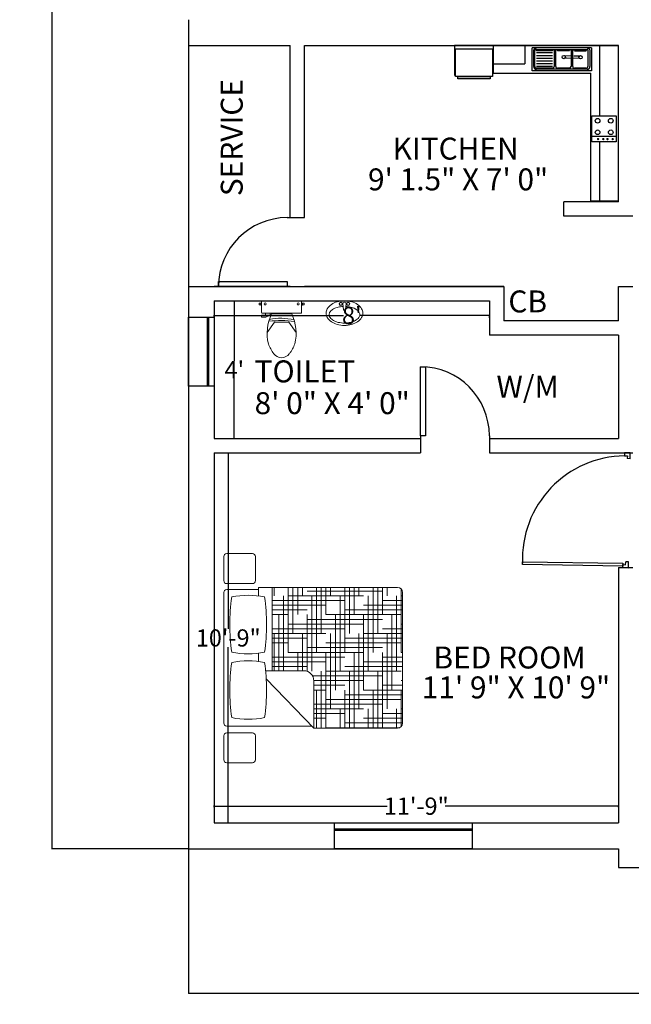
# Model space of a CAD drawing. Units: inches. Extents: x -113 to 5399, y -1393 to 3302.
# Tile 23 of 40: x 3631 to 3844, y -154 to 189. Entities that reach past the tile are written whole.
import ezdxf

# ---------------------------------------------------------------- set-up
doc = ezdxf.new("R2010")
doc.units = ezdxf.units.IN
doc.header["$MEASUREMENT"] = 0
for name, color, linetype, lineweight in [('A-ANNO-DIMS', 254, 'Continuous', 18), ('A-AREA-IDEN', 4, 'Continuous', 18), ('A-FLOR-CASE', 8, 'Continuous', 18), ('A-FLOR-FIXT', 8, 'Continuous', 18), ('doors', 2, 'Continuous', 25), ('DT TEXT', 4, 'Continuous', 18), ('furniture', 131, 'Continuous', 18), ('walls', 1, 'Continuous', 25), ('windows', 3, 'Continuous', 25)]:
    doc.layers.add(name, color=color, linetype=linetype, lineweight=lineweight)
doc.layers.add('A-GLAZ-PATT', color=85, linetype='Continuous', lineweight=13, true_color=0x58ba48)
doc.layers.add('TEFRIŞ', color=11, linetype='Continuous')
doc.styles.get("Standard").update_dxf_attribs({"font": 'arial.ttf'})
doc.dimstyles.get("Standard").update_dxf_attribs({"dimtxt": 6, "dimasz": 0.18, "dimexe": 0.18, "dimexo": 0.0625, "dimgap": 0.09, "dimtad": 0, "dimtih": 1, "dimtoh": 1, "dimdec": 1, "dimzin": 0, "dimdsep": 46, "dimlunit": 4, "dimtxsty": 'Standard', "dimblk": 'ARCHTICK', "dimcen": 0.09, "dimadec": 0, "dimazin": 0, "dimtfac": 1, "dimtdec": 1, "dimtofl": 0, "dimtmove": 0, "dimatfit": 3, "dimfxl": 1, "dimtolj": 1, "dimtzin": 0, "dimarcsym": 0})

# ---------------------------------------------------------------- blocks, each defined once
blk = doc.blocks.new('*U2')
for p, q in [((0, 0), (0, -6)), ((24, 0), (24, -6))]:
    blk.add_line(p, q)
blk.add_lwpolyline([(0, 0), (0, 24), (1.75, 24), (1.75, 0)], close=True)
blk.add_arc((0, 0), 24, 0, 90)
blk = doc.blocks.new('*X4')
at = {"color": 0}
for p, q in [((4.3594, 18.5625), (4.3594, 18.6457)), ((4.5, 18), (4.5, 18.6457)), ((4.5469, 18.1875), (4.5469, 18.6457)), ((4.5938, 18.375), (4.5938, 18.6457)), ((4.6406, 18.5625), (4.6406, 18.6457)), ((4.7812, 18), (4.7812, 18.6457)), ((4.8281, 18.1875), (4.8281, 18.6457)), ((4.875, 18.375), (4.875, 18.6457)), ((4.9219, 18.5625), (4.9219, 18.6457)), ((5.0625, 18), (5.0625, 18.6457)), ((5.1094, 18.1875), (5.1094, 18.6457)), ((5.1562, 18.375), (5.1562, 18.6457)), ((5.2031, 18.5625), (5.2031, 18.6457)), ((5.3438, 18), (5.3438, 18.6457)), ((5.3906, 18.1875), (5.3906, 18.6457)), ((5.4375, 18.375), (5.4375, 18.6457)), ((5.4844, 18.5625), (5.4844, 18.6457)), ((5.625, 18), (5.625, 18.6287)), ((4.4531, 17.8169), (4.4531, 18.5625)), ((4.5, 18.5625), (5.25, 18.5625)), ((4.6875, 18.6094), (5.4375, 18.6094)), ((4.7344, 17.8125), (4.7344, 18.5625)), ((5.0156, 17.8125), (5.0156, 18.5625)), ((5.2969, 17.8125), (5.2969, 18.5625)), ((5.5781, 17.8125), (5.5781, 18.5625)), ((5.625, 18.5625), (5.6375, 18.5625)), ((4.3395, 18.5156), (5.0625, 18.5156)), ((4.3395, 18.4688), (4.875, 18.4688)), ((5.25, 18.4688), (5.6375, 18.4688)), ((5.4375, 18.5156), (5.6375, 18.5156)), ((4.3395, 18.4219), (4.6875, 18.4219)), ((4.3395, 18.375), (4.5, 18.375)), ((4.4062, 17.8169), (4.4062, 18.375)), ((4.6875, 17.8114), (4.6875, 18.375)), ((4.6875, 18.3281), (5.4375, 18.3281)), ((4.875, 18.375), (5.625, 18.375)), ((4.9688, 17.625), (4.9688, 18.375)), ((5.0625, 18.4219), (5.6375, 18.4219)), ((5.25, 17.625), (5.25, 18.375)), ((5.5312, 17.625), (5.5312, 18.375)), ((4.3395, 18.2344), (5.0625, 18.2344)), ((4.5, 18.2812), (5.25, 18.2812)), ((5.4375, 18.2344), (5.6375, 18.2344)), ((5.625, 18.2812), (5.6375, 18.2812)), ((4.3395, 18.1875), (4.875, 18.1875)), ((4.3395, 18.1406), (4.6875, 18.1406)), ((4.3594, 17.8169), (4.3594, 18.1875)), ((4.6406, 17.8169), (4.6406, 18.1875)), ((4.9219, 17.4375), (4.9219, 18.1875)), ((5.0625, 18.1406), (5.6375, 18.1406)), ((5.2031, 17.4375), (5.2031, 18.1875)), ((5.25, 18.1875), (5.6375, 18.1875)), ((5.4844, 17.4375), (5.4844, 18.1875)), ((4.3395, 18.0938), (4.5, 18.0938)), ((4.6875, 18.0469), (5.4375, 18.0469)), ((4.875, 18.0938), (5.625, 18.0938)), ((4.3395, 17.9531), (5.0625, 17.9531)), ((4.5, 18), (5.25, 18)), ((4.5938, 17.8169), (4.5938, 18)), ((4.875, 17.25), (4.875, 18)), ((5.1562, 17.25), (5.1562, 18)), ((5.4375, 17.25), (5.4375, 18)), ((5.4375, 17.9531), (5.6375, 17.9531)), ((5.625, 18), (5.6375, 18)), ((4.3395, 17.9062), (4.875, 17.9062)), ((4.3395, 17.8594), (4.6875, 17.8594)), ((5.0625, 17.8594), (5.6375, 17.8594)), ((5.25, 17.9062), (5.6375, 17.9062)), ((4.7421, 17.7656), (5.4375, 17.7656)), ((4.8281, 17.2457), (4.8281, 17.8125)), ((4.875, 17.8125), (5.625, 17.8125)), ((5.1094, 17.2457), (5.1094, 17.8125)), ((5.3906, 17.2457), (5.3906, 17.8125)), ((4.7548, 17.7188), (5.25, 17.7188)), ((4.7548, 17.6719), (5.0625, 17.6719)), ((5.4375, 17.6719), (5.6375, 17.6719)), ((5.625, 17.7188), (5.6375, 17.7188)), ((4.7548, 17.625), (4.875, 17.625)), ((4.7812, 17.2457), (4.7812, 17.625)), ((5.0625, 17.2457), (5.0625, 17.625)), ((5.0625, 17.5781), (5.6375, 17.5781)), ((5.25, 17.625), (5.6375, 17.625)), ((5.3438, 17.2457), (5.3438, 17.625)), ((5.625, 17.2627), (5.625, 17.625)), ((4.7548, 17.4844), (5.4375, 17.4844)), ((4.875, 17.5312), (5.625, 17.5312)), ((4.7548, 17.4375), (5.25, 17.4375)), ((4.7548, 17.3906), (5.0625, 17.3906)), ((5.0156, 17.2457), (5.0156, 17.4375)), ((5.2969, 17.2457), (5.2969, 17.4375)), ((5.4375, 17.3906), (5.6375, 17.3906)), ((5.5781, 17.2457), (5.5781, 17.4375)), ((5.625, 17.4375), (5.6375, 17.4375)), ((4.7548, 17.3438), (4.875, 17.3438)), ((4.875, 17.25), (5.6077, 17.25)), ((4.9688, 17.2457), (4.9688, 17.25)), ((5.0625, 17.2969), (5.6375, 17.2969)), ((5.25, 17.3438), (5.6375, 17.3438)), ((5.25, 17.2457), (5.25, 17.25)), ((5.5312, 17.2457), (5.5312, 17.25))]:
    blk.add_line(p, q, dxfattribs=at)
blk = doc.blocks.new('MAT-P01')
for p, q in [((-0.0213, 0.8164), (-0.0213, 0.5605)), ((0.0087, 0.8464), (0.2471, 0.8464)), ((0.2771, 0.8164), (0.2771, 0.5605)), ((0.3437, 0.8164), (0.3437, -0.0316)), ((0.3737, 0.8464), (1.6737, 0.8464)), ((1.7037, 0.8164), (1.7037, 0.5005)), ((1.7622, 0.8164), (1.7622, 0.5605)), ((1.7922, 0.8464), (2.0306, 0.8464)), ((2.0606, 0.8164), (2.0606, 0.5605)), ((0.0087, 0.5305), (0.2471, 0.5305)), ((0.9879, 0.5005), (1.0693, 0.5005)), ((1.6393, 0.5005), (1.7237, 0.5005)), ((1.7237, 0.5005), (1.7237, -0.8836)), ((1.7922, 0.5305), (2.0306, 0.5305)), ((0.8146, 0.423), (0.3237, -0.0509)), ((0.8949, 0.4293), (0.8949, 0.0491)), ((0.8949, 0.3643), (1.7237, 0.3643)), ((0.8949, 0.3643), (0.8949, 0.0491)), ((0.8949, 0.3643), (1.7237, 0.3643)), ((1.7237, 0.3643), (1.7237, -0.8836)), ((0.3237, -0.0509), (0.7949, -0.0509)), ((0.3237, -0.0509), (0.3237, -0.8836)), ((0.3737, -0.9336), (1.6737, -0.9336))]:
    blk.add_line(p, q)
for centre, radius, start, end in [((0.0087, 0.8164), 0.03, 90, 180), ((0.2471, 0.8164), 0.03, 0, 90), ((0.3737, 0.8164), 0.03, 90, 180), ((0.7029, -1.1436), 1.9306, 81.81622, 98.18378), ((1.3543, -1.1436), 1.9306, 81.81622, 98.18378), ((1.6737, 0.8164), 0.03, 0, 90), ((1.7922, 0.8164), 0.03, 90, 180), ((2.0306, 0.8164), 0.03, 0, 90), ((1.2251, 0.6034), 0.8138, 168.37298, 191.62702), ((0.1806, 0.6034), 0.8138, 348.37298, 11.62702), ((1.8766, 0.6034), 0.8138, 168.37298, 191.62702), ((0.8321, 0.6034), 0.8138, 348.37298, 11.62702), ((0.0087, 0.5605), 0.03, 180, 270), ((0.2471, 0.5605), 0.03, 270, 0), ((1.7922, 0.5605), 0.03, 180, 270), ((2.0306, 0.5605), 0.03, 270, 0), ((0.7029, 2.3504), 1.9306, 261.81622, 278.18378), ((1.3543, 2.3504), 1.9306, 261.81622, 278.18378), ((0.7949, 0.0491), 0.1, 270, 0), ((0.3737, -0.8836), 0.05, 180, 270), ((1.6737, -0.8836), 0.05, 270, 0)]:
    blk.add_arc(centre, radius, start, end)
at = {"rotation": 270}
blk.add_blockref('*X4', (-16.9221, 4.7038), dxfattribs=at)
blk = doc.blocks.new('A$C008029BD')
at = {"layer": 'TEFRIŞ', "ltscale": 0.05}
for p, q in [((0, 0), (0, -3.55)), ((3.37, 0), (0, 0)), ((3.37, 0), (3.37, -0.6)), ((1.522, -0.4), (0, -0.4)), ((3.37, -0.4), (2.083, -0.4)), ((0.05, -0.581), (0.05, -1.869)), ((0.05, -0.581), (0.55, -0.581)), ((0.096, -0.617), (0.454, -0.617)), ((0.55, -0.581), (0.55, -1.869)), ((0.6, -2.71), (0.6, -0.6)), ((3.37, -0.6), (0.6, -0.6)), ((0.086, -1.773), (0.086, -0.677)), ((0.099, -0.659), (0.457, -0.659)), ((0.113, -0.954), (0.113, -0.695)), ((0.23, -0.846), (0.229, -0.967)), ((0.28, -0.846), (0.277, -1.158)), ((0.493, -0.695), (0.493, -0.954)), ((0.514, -0.677), (0.514, -1.773)), ((0.096, -1.024), (0.454, -1.024)), ((0.457, -0.99), (0.099, -0.99)), ((0.11, -1.319), (0.11, -1.06)), ((0.228, -1.02), (0.227, -1.159)), ((0.49, -1.06), (0.49, -1.319)), ((0.454, -1.355), (0.096, -1.355)), ((0.096, -1.391), (0.454, -1.391)), ((0.11, -1.773), (0.11, -1.427)), ((0.154, -1.773), (0.154, -1.427)), ((0.214, -1.773), (0.214, -1.427)), ((0.274, -1.773), (0.274, -1.427)), ((0.334, -1.773), (0.334, -1.427)), ((0.39, -1.773), (0.39, -1.427)), ((0.444, -1.773), (0.444, -1.427)), ((0.49, -1.427), (0.49, -1.773)), ((0.55, -1.869), (0.05, -1.869)), ((0.454, -1.809), (0.096, -1.809)), ((0.454, -1.833), (0.096, -1.833)), ((0, -2.025), (0.4, -2.025)), ((0.4, -2.71), (0.4, -2.025)), ((0, -2.71), (0.6, -2.71)), ((0, -3.55), (0.65, -3.55))]:
    blk.add_line(p, q, dxfattribs=at)
at = {"layer": 'TEFRIŞ'}
blk.add_line((1.969, -0.05), (1.969, -0.572), dxfattribs=at)
at = {"layer": 'TEFRIŞ', "ltscale": 0.05}
for points in [[(1.522, -0.05), (2.083, -0.05), (2.083, -0.572), (1.522, -0.572)], [(0.67, -2.73), (0.67, -3.53), (0.07, -3.53), (0.07, -2.73)], [(0.72, -2.78), (0.72, -3.48), (0.67, -3.48), (0.67, -2.78)]]:
    blk.add_lwpolyline(points, close=True, dxfattribs=at)
at = {"layer": 'TEFRIŞ', "const_width": 0.025}
for points in [[(2.014, -0.123, 1), (2.039, -0.123, 1)], [(2.014, -0.236, 1), (2.039, -0.236, 1)], [(2.014, -0.327, 1), (2.039, -0.327, 1)], [(2.014, -0.44, 1), (2.039, -0.44, 1)]]:
    blk.add_lwpolyline(points, format="xyb", close=True, dxfattribs=at)
at = {"layer": 'TEFRIŞ', "ltscale": 0.05}
for centre, radius in [((1.628, -0.164), 0.0505), ((1.628, -0.45), 0.0505), ((0.255, -0.82), 0.036), ((0.252, -1.184), 0.036)]:
    blk.add_circle(centre, radius, dxfattribs=at)
at = {"layer": 'TEFRIŞ'}
for centre in [(1.88, -0.164), (1.88, -0.45)]:
    blk.add_circle(centre, 0.0505, dxfattribs=at)
at = {"layer": 'TEFRIŞ', "ltscale": 0.05}
for centre, radius, start, end in [((0.108, -0.649), 0.0351, 110.4976, 230.5777), ((0.454, -0.677), 0.06, 0, 90), ((0.118, -0.673), 0.023, 143.9853, 258.5157), ((0.457, -0.695), 0.036, 0, 90), ((0.115, -1.038), 0.023, 143.9853, 258.5157), ((0.118, -0.976), 0.023, 101.4843, 216.0147), ((0.454, -1.06), 0.036, 0, 90), ((0.457, -0.954), 0.036, 270, 0), ((0.115, -1.341), 0.023, 101.4843, 216.0147), ((0.115, -1.405), 0.023, 143.9853, 258.5157), ((0.454, -1.319), 0.036, 270, 0), ((0.454, -1.427), 0.036, 0, 90), ((0.108, -1.801), 0.0351, 129.4223, 249.5024), ((0.115, -1.796), 0.023, 101.4843, 216.0147), ((0.454, -1.773), 0.06, 270, 0), ((0.454, -1.773), 0.036, 270, 0)]:
    blk.add_arc(centre, radius, start, end, dxfattribs=at)
blk = doc.blocks.new('toilet-3')
at = {"color": 0, "linetype": 'ByBlock'}
for p, q in [((-0.281, -0.05), (-0.281, -0.069)), ((-0.281, -0.05), (-0.261, -0.05)), ((-0.281, -0.069), (-0.261, -0.069)), ((-0.261, -0.047), (-0.261, -0.072)), ((-0.261, -0.047), (-0.251, -0.047)), ((-0.261, -0.072), (-0.251, -0.072)), ((-0.251, -0.047), (-0.251, -0.072)), ((-0.25, -0.03), (-0.25, -0.165)), ((0.24, -0.02), (-0.24, -0.02)), ((0.25, -0.03), (0.25, -0.165)), ((0.261, -0.047), (0.251, -0.047)), ((0.251, -0.047), (0.251, -0.072)), ((0.261, -0.072), (0.251, -0.072)), ((0.261, -0.047), (0.261, -0.072)), ((0.281, -0.05), (0.261, -0.05)), ((0.281, -0.069), (0.261, -0.069)), ((0.281, -0.05), (0.281, -0.069)), ((-0.144, -0.2), (-0.25, -0.2)), ((-0.25, -0.2), (-0.25, -0.222)), ((-0.198, -0.222), (-0.25, -0.222)), ((0.24, -0.175), (-0.24, -0.175)), ((-0.202, -0.2), (-0.202, -0.175)), ((-0.198, -0.222), (-0.16, -0.207)), ((-0.16, -0.207), (-0.16, -0.2)), ((-0.144, -0.2), (-0.144, -0.175)), ((0.125, -0.182), (-0.125, -0.182)), ((-0.089, -0.287), (-0.18, -0.415)), ((0.089, -0.287), (-0.089, -0.287)), ((0.089, -0.287), (0.18, -0.415))]:
    blk.add_line(p, q, dxfattribs=at)
for centre in [(-0.205, -0.059), (0.205, -0.059)]:
    blk.add_circle(centre, 0.0125, dxfattribs=at)
for centre, radius, start, end in [((-0.24, -0.03), 0.01, 90, 180), ((0.24, -0.03), 0.01, 0, 90), ((-0.24, -0.165), 0.01, 180, 270), ((0.376, -0.424), 0.557, 154.2321, 193.6755), ((-0.005, -0.896), 0.659, 75.9276, 103.0204), ((-0.376, -0.424), 0.557, 346.3245, 25.7679), ((0.24, -0.165), 0.01, 270, 0), ((-0.013, -1.787), 1.521, 83.4552, 95.5271), ((0.262, -0.406), 0.452, 199.2942, 217.2549), ((-0.265, -0.4), 0.457, 322.2382, 340.1051), ((-0.001, -0.609), 0.12, 216.3794, 323.6206)]:
    blk.add_arc(centre, radius, start, end, dxfattribs=at)
blk = doc.blocks.new('wash-6')
at = {"color": 0, "linetype": 'ByBlock'}
for p, q in [((-0.036, -0.063), (-0.021, -0.18)), ((0.036, -0.063), (0.021, -0.18))]:
    blk.add_line(p, q, dxfattribs=at)
for centre, radius in [((-0.075, -0.062), 0.0325), ((-0.075, -0.062), 0.0263), ((0.075, -0.062), 0.0325), ((0.075, -0.062), 0.0263)]:
    blk.add_circle(centre, radius, dxfattribs=at)
for centre, radius, start, end in [((0, -0.56), 0.56, 90, 105.4371), ((-0.204, -0.25), 0.17, 148.1465, 180), ((-0.107, -0.311), 0.285, 123.6901, 148.1465), ((-0.114, -0.361), 0.225, 118.369, 142.5096), ((-0.042, -0.407), 0.401, 105.4371, 123.6901), ((-0.045, -0.488), 0.37, 102.6081, 118.369), ((0, -0.69), 0.576, 92.9466, 102.6081), ((0, -0.063), 0.0361, 0, 180), ((0, -0.18), 0.0215, 180, 0), ((0, -0.56), 0.56, 74.5629, 90), ((0, -0.69), 0.576, 77.3919, 87.0534), ((0.045, -0.488), 0.37, 61.631, 77.3919), ((0.042, -0.407), 0.401, 56.3099, 74.5629), ((0.114, -0.361), 0.225, 37.4904, 61.631), ((0.107, -0.311), 0.285, 31.8535, 56.3099), ((0.204, -0.25), 0.17, 0, 31.8535), ((-0.204, -0.25), 0.17, 180, 211.8535), ((-0.107, -0.189), 0.285, 211.8535, 236.3099), ((-0.217, -0.282), 0.0954, 142.5096, 180), ((-0.217, -0.282), 0.0954, 180, 217.4904), ((-0.114, -0.203), 0.225, 217.4904, 241.631), ((0.114, -0.203), 0.225, 298.369, 322.5096), ((0.107, -0.189), 0.285, 303.6901, 328.1465), ((0.217, -0.282), 0.0954, 0, 37.4904), ((0.217, -0.282), 0.0954, 322.5096, 0), ((0.204, -0.25), 0.17, 328.1465, 0), ((-0.042, -0.092), 0.401, 236.3099, 254.5629), ((-0.045, -0.076), 0.37, 241.631, 257.3919), ((0, 0.06), 0.56, 254.5629, 270), ((0, 0.125), 0.576, 257.3919, 270), ((0, 0.125), 0.576, 270, 282.6081), ((0, 0.06), 0.56, 270, 285.4371), ((0.045, -0.076), 0.37, 282.6081, 298.369), ((0.042, -0.092), 0.401, 285.4371, 303.6901)]:
    blk.add_arc(centre, radius, start, end, dxfattribs=at)
blk = doc.blocks.new('_ArchTick')
at = {"color": 0, "linetype": 'ByBlock', "const_width": 0.15}
blk.add_lwpolyline([(-0.5, -0.5), (0.5, 0.5)], dxfattribs=at)
blk = doc.blocks.new('*D99')
at = {"layer": 'A-ANNO-DIMS', "color": 0, "lineweight": -2, "transparency": 16777216}
for p, q in [((3689.73, -100.29), (3689.73, -150.66)), ((4122.73, -100.29), (4122.73, -150.66)), ((3689.73, -150.48), (3895.84, -150.48)), ((4122.73, -150.48), (3916.62, -150.48))]:
    blk.add_line(p, q, dxfattribs=at)
at = {"layer": 'Defpoints', "color": 0, "transparency": 16777216}
for p in [(3689.73, -100.22), (4122.73, -100.22), (4122.73, -150.48)]:
    blk.add_point(p, dxfattribs=at)
at = {"layer": 'A-ANNO-DIMS', "color": 0, "lineweight": -2, "transparency": 16777216, "xscale": 0.18, "yscale": 0.18, "zscale": 0.18, "rotation": 180}
blk.add_blockref('_ArchTick', (3689.73, -150.48), dxfattribs=at)
at = {"layer": 'A-ANNO-DIMS', "color": 0, "lineweight": -2, "transparency": 16777216, "xscale": 0.18, "yscale": 0.18, "zscale": 0.18}
blk.add_blockref('_ArchTick', (4122.73, -150.48), dxfattribs=at)
at = {"layer": 'A-ANNO-DIMS', "color": 0, "transparency": 16777216, "insert": (3906.23, -150.48), "char_height": 6, "attachment_point": 5}
blk.add_mtext('\\A1;36\'-1"', dxfattribs=at)
blk = doc.blocks.new('*D100')
at = {"layer": 'A-ANNO-DIMS', "color": 0, "lineweight": -2, "transparency": 16777216}
for p, q in [((3689.67, 549.78), (3642.02, 549.78)), ((3642.2, 549.78), (3642.2, 227.93)), ((3642.2, -100.22), (3642.2, 221.62)), ((3689.67, -100.22), (3642.02, -100.22))]:
    blk.add_line(p, q, dxfattribs=at)
at = {"layer": 'Defpoints', "color": 0, "transparency": 16777216}
for p in [(3689.73, 549.78), (3642.2, -100.22), (3689.73, -100.22)]:
    blk.add_point(p, dxfattribs=at)
at = {"layer": 'A-ANNO-DIMS', "color": 0, "lineweight": -2, "transparency": 16777216, "xscale": 0.18, "yscale": 0.18, "zscale": 0.18}
for p, rotation in [((3642.2, 549.78), 90), ((3642.2, -100.22), 270)]:
    blk.add_blockref('_ArchTick', p, dxfattribs=dict(at, rotation=rotation))
at = {"layer": 'A-ANNO-DIMS', "color": 0, "transparency": 16777216, "insert": (3642.2, 224.78), "char_height": 6, "attachment_point": 5}
blk.add_mtext('\\A1;54\'-2"', dxfattribs=at)
blk = doc.blocks.new('*D107')
at = {"layer": 'A-ANNO-DIMS', "color": 0, "lineweight": -2, "transparency": 16777216}
for p, q in [((3703.08, 37.78), (3703.82, 37.78)), ((3703.64, 37.78), (3703.64, -23.57)), ((3703.64, -91.22), (3703.64, -29.88)), ((3703.08, -91.22), (3703.82, -91.22))]:
    blk.add_line(p, q, dxfattribs=at)
at = {"layer": 'Defpoints', "color": 0, "transparency": 16777216}
for p in [(3703.02, 37.78), (3703.02, -91.22), (3703.64, -91.22)]:
    blk.add_point(p, dxfattribs=at)
at = {"layer": 'A-ANNO-DIMS', "color": 0, "lineweight": -2, "transparency": 16777216, "xscale": 0.18, "yscale": 0.18, "zscale": 0.18}
for p, rotation in [((3703.64, 37.78), 90), ((3703.64, -91.22), 270)]:
    blk.add_blockref('_ArchTick', p, dxfattribs=dict(at, rotation=rotation))
at = {"layer": 'A-ANNO-DIMS', "color": 0, "transparency": 16777216, "insert": (3703.64, -26.72), "char_height": 6, "attachment_point": 5}
blk.add_mtext('\\A1;10\'-9"', dxfattribs=at)
blk = doc.blocks.new('*D108')
at = {"layer": 'A-ANNO-DIMS', "color": 0, "lineweight": -2, "transparency": 16777216}
for p, q in [((3698.73, -85.71), (3698.73, -85.17)), ((3698.73, -85.35), (3759.12, -85.35)), ((3839.73, -85.35), (3779.34, -85.35)), ((3839.73, -85.71), (3839.73, -85.17))]:
    blk.add_line(p, q, dxfattribs=at)
at = {"layer": 'Defpoints', "color": 0, "transparency": 16777216}
for p in [(3698.73, -85.77), (3839.73, -85.35), (3839.73, -85.77)]:
    blk.add_point(p, dxfattribs=at)
at = {"layer": 'A-ANNO-DIMS', "color": 0, "lineweight": -2, "transparency": 16777216, "xscale": 0.18, "yscale": 0.18, "zscale": 0.18, "rotation": 180}
blk.add_blockref('_ArchTick', (3698.73, -85.35), dxfattribs=at)
at = {"layer": 'A-ANNO-DIMS', "color": 0, "lineweight": -2, "transparency": 16777216, "xscale": 0.18, "yscale": 0.18, "zscale": 0.18}
blk.add_blockref('_ArchTick', (3839.73, -85.35), dxfattribs=at)
at = {"layer": 'A-ANNO-DIMS', "color": 0, "transparency": 16777216, "insert": (3769.23, -85.35), "char_height": 6, "attachment_point": 5}
blk.add_mtext('\\A1;11\'-9"', dxfattribs=at)
blk = doc.blocks.new('*D117')
at = {"layer": 'A-ANNO-DIMS', "color": 0, "lineweight": -2, "transparency": 16777216}
for p, q in [((3705.76, 90.78), (3705.76, 69.87)), ((3705.83, 90.78), (3705.94, 90.78)), ((3705.76, 42.78), (3705.76, 63.69)), ((3705.83, 42.78), (3705.94, 42.78))]:
    blk.add_line(p, q, dxfattribs=at)
at = {"layer": 'Defpoints', "color": 0, "transparency": 16777216}
for p in [(3705.76, 90.78), (3705.76, 42.78), (3705.76, 42.78)]:
    blk.add_point(p, dxfattribs=at)
at = {"layer": 'A-ANNO-DIMS', "color": 0, "lineweight": -2, "transparency": 16777216, "xscale": 0.18, "yscale": 0.18, "zscale": 0.18}
for p, rotation in [((3705.76, 90.78), 90), ((3705.76, 42.78), 270)]:
    blk.add_blockref('_ArchTick', p, dxfattribs=dict(at, rotation=rotation))
at = {"layer": 'A-ANNO-DIMS', "color": 0, "transparency": 16777216, "insert": (3705.76, 66.78), "char_height": 6, "attachment_point": 5}
blk.add_mtext("\\A1;4'", dxfattribs=at)
blk = doc.blocks.new('*D118')
at = {"layer": 'A-ANNO-DIMS', "color": 0, "lineweight": -2, "transparency": 16777216}
for p, q in [((3698.73, 84.84), (3698.73, 85.81)), ((3794.73, 84.84), (3794.73, 85.81)), ((3698.73, 85.63), (3743.87, 85.63)), ((3794.73, 85.63), (3749.58, 85.63))]:
    blk.add_line(p, q, dxfattribs=at)
at = {"layer": 'Defpoints', "color": 0, "transparency": 16777216}
for p in [(3698.73, 85.63), (3698.73, 84.78), (3794.73, 84.78)]:
    blk.add_point(p, dxfattribs=at)
at = {"layer": 'A-ANNO-DIMS', "color": 0, "lineweight": -2, "transparency": 16777216, "xscale": 0.18, "yscale": 0.18, "zscale": 0.18, "rotation": 180}
blk.add_blockref('_ArchTick', (3698.73, 85.63), dxfattribs=at)
at = {"layer": 'A-ANNO-DIMS', "color": 0, "lineweight": -2, "transparency": 16777216, "xscale": 0.18, "yscale": 0.18, "zscale": 0.18}
blk.add_blockref('_ArchTick', (3794.73, 85.63), dxfattribs=at)
at = {"layer": 'A-ANNO-DIMS', "color": 0, "transparency": 16777216, "insert": (3746.73, 85.63), "char_height": 6, "attachment_point": 5}
blk.add_mtext("\\A1;8'", dxfattribs=at)
blk = doc.blocks.new('WIN-PLAN-48IN')
h = blk.add_hatch(color=256)
h.dxf.hatch_style = 1
h.paths.add_polyline_path([(48, 2.5), (0, 2.5), (0, 2), (48, 2)])
for p, q in [((0, 9), (48, 9)), ((0, 0), (0, 9)), ((48, 9), (48, 0)), ((48, 2.5), (0, 2.5)), ((48, 2), (0, 2)), ((48, 0), (0, 0))]:
    blk.add_line(p, q)
blk = doc.blocks.new('DOOR-SINGLE-36IN-PLAN')
for p, q in [((0.5, 2), (0.5, 36.98)), ((0.5, 36.98), (1.5, 36.98)), ((1.5, 36.98), (1.5, 2)), ((0, 2), (0, 0)), ((0, 2), (1.04, 2)), ((1.5, 2), (0.5, 2)), ((1.04, 2), (1.04, 0.98)), ((1.04, 0.98), (2, 0.98)), ((2, 0), (2, 0.98)), ((38.96, 0.98), (38, 0.98)), ((38, 0), (38, 0.98)), ((40, 2), (38.96, 2)), ((38.96, 2), (38.96, 0.98)), ((40, 0), (40, 2)), ((0, 0), (2, 0)), ((0, 0), (2, 0)), ((38, 0), (40, 0))]:
    blk.add_line(p, q)
blk.add_arc((2.94, 0.99), 36.04, 1.6003, 93.0893)
blk = doc.blocks.new('*D210')
at = {"layer": 'A-ANNO-DIMS', "color": 0, "lineweight": -2, "transparency": 16777216}
for p, q in [((3839.79, 561.28), (4159.21, 561.28)), ((4159.03, 561.28), (4159.03, 230.43)), ((4159.03, -106.72), (4159.03, 224.12)), ((3839.79, -106.72), (4159.21, -106.72))]:
    blk.add_line(p, q, dxfattribs=at)
at = {"layer": 'Defpoints', "color": 0, "transparency": 16777216}
for p in [(3839.73, 561.28), (4159.03, 561.28), (3839.73, -106.72)]:
    blk.add_point(p, dxfattribs=at)
at = {"layer": 'A-ANNO-DIMS', "color": 0, "lineweight": -2, "transparency": 16777216, "xscale": 0.18, "yscale": 0.18, "zscale": 0.18}
for p, rotation in [((4159.03, 561.28), 90), ((4159.03, -106.72), 270)]:
    blk.add_blockref('_ArchTick', p, dxfattribs=dict(at, rotation=rotation))
at = {"layer": 'A-ANNO-DIMS', "color": 0, "transparency": 16777216, "insert": (4159.03, 227.28), "char_height": 6, "attachment_point": 5}
blk.add_mtext('\\A1;55\'-8"', dxfattribs=at)

msp = doc.modelspace()

# ---------------------------------------------------------------- hatches: boundary and pattern name
at = {"layer": 'A-GLAZ-PATT'}
h = msp.add_hatch(color=256, dxfattribs=at)
h.dxf.hatch_style = 1
h.paths.add_polyline_path([(3696.23, 85.06), (3696.23, 61.06), (3696.73, 61.06), (3696.73, 85.06)])

# ---------------------------------------------------------------- linework, layer by layer
at = {"layer": 'walls'}
for p, q in [((3689.73, 188.78), (3689.73, -100.22)), ((3689.73, 179.78), (3725.23, 179.78)), ((3725.23, 119.78), (3725.23, 179.78)), ((3730.23, 119.78), (3730.23, 179.78)), ((3730.23, 179.78), (3839.73, 179.78)), ((3839.73, 125.28), (3839.73, 179.78)), ((3839.73, 125.28), (3820.73, 125.28)), ((3820.73, 120.28), (3820.73, 125.28)), ((3844.73, 120.28), (3820.73, 120.28)), ((3725.23, 119.78), (3730.23, 119.78)), ((3689.73, 95.78), (3725.23, 95.78)), ((3725.23, 95.78), (3698.73, 95.78)), ((3725.23, 95.78), (3730.23, 95.78)), ((3799.73, 95.78), (3730.23, 95.78)), ((3730.23, 95.78), (3799.73, 95.78)), ((3799.73, 95.78), (3799.73, 83.78)), ((3839.73, 83.78), (3839.73, 95.78)), ((3839.73, 95.78), (3844.73, 95.78)), ((3698.73, 90.78), (3698.73, 42.78)), ((3698.73, 90.78), (3794.73, 90.78)), ((3698.73, 90.78), (3794.73, 90.78)), ((3794.73, 90.78), (3794.73, 78.78)), ((3839.73, 83.78), (3799.73, 83.78)), ((3839.73, 78.78), (3794.73, 78.78)), ((3839.73, 78.78), (3839.73, 42.78)), ((3698.73, 42.78), (3770.73, 42.78)), ((3770.73, 42.78), (3770.73, 37.78)), ((3794.73, 43.78), (3794.73, 37.78)), ((3794.73, 42.78), (3839.73, 42.78)), ((3698.73, 37.78), (3698.73, -91.22)), ((3698.73, 37.78), (3770.73, 37.78)), ((3794.73, 37.78), (3839.73, 37.78)), ((3839.73, 37.78), (3844.73, 37.78)), ((3839.73, -2.22), (3839.73, -91.22)), ((3839.73, -2.22), (3844.73, -2.22)), ((3698.73, -91.22), (3839.73, -91.22)), ((3689.73, -100.22), (3839.73, -100.22)), ((3839.73, -100.22), (3839.73, -106.72)), ((3839.73, -106.72), (3844.73, -106.72))]:
    msp.add_line(p, q, dxfattribs=at)
at = {"layer": 'windows'}
for p, q in [((3689.73, 61.06), (3689.73, 85.06)), ((3689.73, 85.06), (3698.73, 85.06)), ((3696.23, 85.06), (3696.23, 61.06)), ((3696.73, 85.06), (3696.73, 61.06)), ((3698.73, 85.06), (3698.73, 61.06)), ((3698.73, 61.06), (3689.73, 61.06))]:
    msp.add_line(p, q, dxfattribs=at)

# ---------------------------------------------------------------- block references
at = {"layer": 'A-FLOR-CASE', "xscale": 16.09806929200166, "yscale": 16.09806929200166, "zscale": 16.09806929200166, "rotation": 270}
msp.add_blockref('A$C008029BD', (3839.73, 179.78), dxfattribs=at)
at = {"layer": 'A-FLOR-FIXT'}
for name, p, xscale, yscale, zscale in [('toilet-3', (3722.26, 91.34), 27.95492935005888, 27.95492935005888, 27.95492935005888), ('wash-6', (3744.18, 90.78), 17.16666334294967, 17.16666334294967, 17.16666334294967)]:
    msp.add_blockref(name, p, dxfattribs=dict(at, xscale=xscale, yscale=yscale, zscale=zscale))
at = {"layer": 'doors'}
for name, p, rotation in [('*U2', (3724.23, 95.78), 90.00000000000003), ('DOOR-SINGLE-36IN-PLAN', (3843.23, -2.24), 89.09244041659026)]:
    msp.add_blockref(name, p, dxfattribs=dict(at, rotation=rotation))
msp.add_blockref('*U2', (3770.73, 43.78), dxfattribs=at)
at = {"layer": 'furniture', "xscale": 35.02364872074636, "yscale": 35.02364872074636, "zscale": 35.02364872074636, "rotation": 90}
msp.add_blockref('MAT-P01', (3731.72, -69.49), dxfattribs=at)
at = {"layer": 'windows', "rotation": 180}
msp.add_blockref('WIN-PLAN-48IN', (3788.73, -91.22), dxfattribs=at)

# ---------------------------------------------------------------- texts
at = {"layer": 'A-AREA-IDEN'}
msp.add_text('SERVICE', height=7.647, rotation=90, dxfattribs=at).set_placement((3708.68, 127.27))
for s, height, p in [('KITCHEN', 7.647, (3760.98, 140.01)), ('9\' 1.5" X 7\' 0"', 7.6473, (3752.39, 129.29)), ('TOILET', 7.647, (3712.82, 62.37)), ('8\' 0" X 4\' 0"', 7.6473, (3712.82, 51.29)), ('BED ROOM', 7.647, (3775.23, -37.37)), ('11\' 9" X 10\' 9"', 7.6473, (3771.13, -47.79))]:
    msp.add_text(s, height=height, dxfattribs=at).set_placement(p)
at = {"layer": 'DT TEXT'}
for s, p in [('CB', (3801.35, 86.75)), (' W/M', (3794.88, 57))]:
    msp.add_text(s, height=7.647, dxfattribs=at).set_placement(p)

# ---------------------------------------------------------------- dimensions: what is measured, and where the dimension line sits
at = {"layer": 'A-ANNO-DIMS'}
for base, p1, p2, override, picture, middle in [((4159.03, 561.28), (3839.73, -106.72), (3839.73, 561.28), {"dimdec": 1, "dimlfac": 1, "dimrnd": 0, "dimzin": 1, "dimdsep": 46, "dimlunit": 4, "dimfrac": 2}, '*D210', (4159.03, 227.28)), ((3642.2, -100.22), (3689.73, 549.78), (3689.73, -100.22), {"dimclrd": 0, "dimclre": 0, "dimclrt": 0}, '*D100', (3642.2, 224.78)), ((3705.76, 42.78), (3705.76, 90.78), (3705.76, 42.78), {"dimclrd": 0, "dimclre": 0, "dimclrt": 0}, '*D117', (3705.76, 66.78)), ((3703.64, -91.22), (3703.02, 37.78), (3703.02, -91.22), {"dimclrd": 0, "dimclre": 0, "dimclrt": 0}, '*D107', (3703.64, -26.72))]:
    dim = msp.add_linear_dim(base=base, p1=p1, p2=p2, angle=90, dimstyle='Standard', override=override, dxfattribs=at)
    dim.commit()
    dim.dimension.update_dxf_attribs({"geometry": picture, "text_midpoint": middle})
for base, p1, p2, picture, middle in [((3698.73, 85.63), (3794.73, 84.78), (3698.73, 84.78), '*D118', (3746.73, 85.63)), ((3839.73, -85.35), (3698.73, -85.77), (3839.73, -85.77), '*D108', (3769.23, -85.35)), ((4122.73, -150.48), (3689.73, -100.22), (4122.73, -100.22), '*D99', (3906.23, -150.48))]:
    dim = msp.add_linear_dim(base=base, p1=p1, p2=p2, dimstyle='Standard', override={"dimclrd": 0, "dimclre": 0, "dimclrt": 0}, dxfattribs=at)
    dim.commit()
    dim.dimension.update_dxf_attribs({"geometry": picture, "text_midpoint": middle})

doc.saveas('drawing.dxf')
